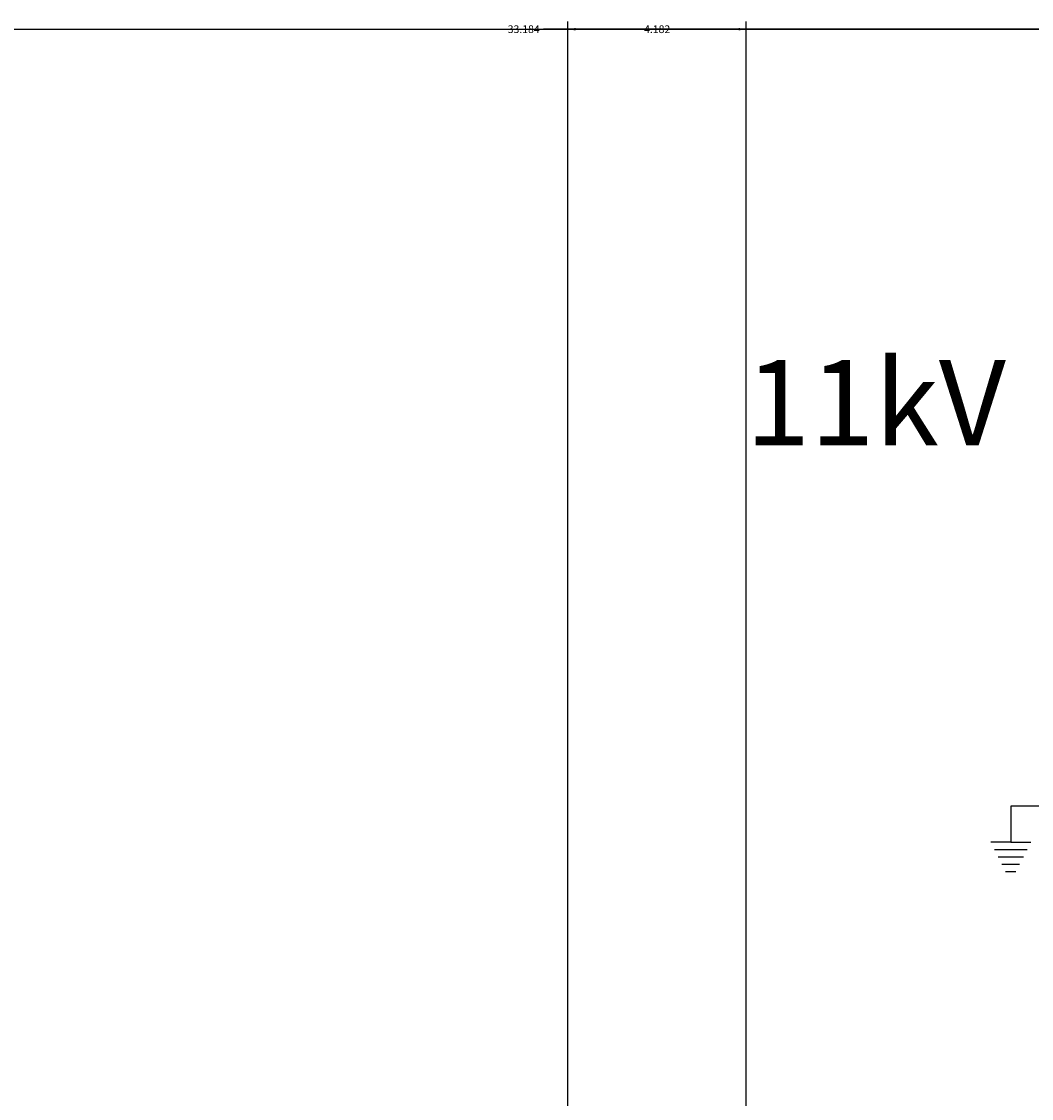
# Model space of a CAD drawing. Units: inches. Extents: x 412 to 584, y 208 to 437.
# Tile 24 of 28: x 471 to 495, y 412 to 437. Entities that reach past the tile are written whole.
import ezdxf

# ---------------------------------------------------------------- set-up
doc = ezdxf.new("R2010")
doc.units = ezdxf.units.IN
doc.header["$MEASUREMENT"] = 0
for name, color, linetype, lineweight in [('A-ANNO-DIMS', 2, 'Continuous', 18), ('E-ANNO-TEXT', 7, 'Continuous', 18), ('E-POWR-EQPM', 3, 'Continuous', 25)]:
    doc.layers.add(name, color=color, linetype=linetype, lineweight=lineweight)
doc.styles.get("Standard").update_dxf_attribs({"font": 'arial.ttf'})
doc.dimstyles.get("Standard").update_dxf_attribs({"dimtxt": 0.18, "dimasz": 0.18, "dimexe": 0.18, "dimexo": 0.0625, "dimgap": 0.09, "dimtad": 0, "dimtih": 1, "dimtoh": 1, "dimdec": 4, "dimzin": 0, "dimdsep": 46, "dimtxsty": 'Standard', "dimcen": 0.09, "dimadec": 0, "dimazin": 0, "dimtfac": 1, "dimtdec": 4, "dimtofl": 0, "dimtmove": 0, "dimatfit": 3, "dimfxl": 1, "dimtolj": 1, "dimtzin": 0, "dimarcsym": 0})

# ---------------------------------------------------------------- blocks, each defined once
blk = doc.blocks.new('*D21')
at = {"layer": 'A-ANNO-DIMS', "color": 0, "lineweight": -2, "transparency": 16777216}
for p, q in [((466.104, 400.237), (466.104, 437.465)), ((538.619, 400.237), (538.619, 437.465)), ((466.284, 437.285), (501.986, 437.285)), ((538.439, 437.285), (502.737, 437.285))]:
    blk.add_line(p, q, dxfattribs=at)
at = {"layer": 'A-ANNO-DIMS', "color": 0, "transparency": 16777216}
for points in [[(466.284, 437.315), (466.284, 437.255), (466.104, 437.285)], [(538.439, 437.315), (538.439, 437.255), (538.619, 437.285)]]:
    blk.add_solid(points, dxfattribs=at)
at = {"layer": 'Defpoints', "color": 0, "transparency": 16777216}
for p in [(538.619, 437.285), (466.104, 400.175), (538.619, 400.175)]:
    blk.add_point(p, dxfattribs=at)
at = {"layer": 'A-ANNO-DIMS', "color": 0, "transparency": 16777216, "insert": (502.361, 437.285), "char_height": 0.18, "attachment_point": 5}
blk.add_mtext('\\A1;72.51', dxfattribs=at)
blk = doc.blocks.new('*D27')
at = {"layer": 'A-ANNO-DIMS', "color": 0, "lineweight": -2, "transparency": 16777216}
for p, q in [((466.104, 400.237), (466.104, 437.465)), ((499.288, 397.825), (499.288, 437.465)), ((466.284, 437.285), (482.233, 437.285)), ((499.108, 437.285), (483.159, 437.285))]:
    blk.add_line(p, q, dxfattribs=at)
at = {"layer": 'A-ANNO-DIMS', "color": 0, "transparency": 16777216}
for points in [[(466.284, 437.315), (466.284, 437.255), (466.104, 437.285)], [(499.108, 437.315), (499.108, 437.255), (499.288, 437.285)]]:
    blk.add_solid(points, dxfattribs=at)
at = {"layer": 'Defpoints', "color": 0, "transparency": 16777216}
for p in [(499.288, 437.285), (466.104, 400.175), (499.288, 397.763)]:
    blk.add_point(p, dxfattribs=at)
at = {"layer": 'A-ANNO-DIMS', "color": 0, "transparency": 16777216, "insert": (482.696, 437.285), "char_height": 0.18, "attachment_point": 5}
blk.add_mtext('\\A1;33.184', dxfattribs=at)
blk = doc.blocks.new('*D28')
at = {"layer": 'A-ANNO-DIMS', "color": 0, "lineweight": -2, "transparency": 16777216}
for p, q in [((450.562, 256.635), (450.562, 437.465)), ((555.796, 256.635), (555.796, 437.465)), ((450.742, 437.285), (502.724, 437.285)), ((555.616, 437.285), (503.634, 437.285))]:
    blk.add_line(p, q, dxfattribs=at)
at = {"layer": 'A-ANNO-DIMS', "color": 0, "transparency": 16777216}
for points in [[(450.742, 437.315), (450.742, 437.255), (450.562, 437.285)], [(555.616, 437.315), (555.616, 437.255), (555.796, 437.285)]]:
    blk.add_solid(points, dxfattribs=at)
at = {"layer": 'Defpoints', "color": 0, "transparency": 16777216}
for p in [(555.796, 437.285), (450.562, 256.573), (555.796, 256.573)]:
    blk.add_point(p, dxfattribs=at)
at = {"layer": 'A-ANNO-DIMS', "color": 0, "transparency": 16777216, "insert": (503.179, 437.285), "char_height": 0.18, "attachment_point": 5}
blk.add_mtext('\\A1;105.23', dxfattribs=at)
blk = doc.blocks.new('*D41')
at = {"layer": 'A-ANNO-DIMS', "color": 0, "lineweight": -2, "transparency": 16777216}
for p, q in [((483.735, 316.045), (483.735, 437.465)), ((487.917, 316.045), (487.917, 437.465)), ((483.915, 437.285), (485.429, 437.285)), ((487.737, 437.285), (486.222, 437.285))]:
    blk.add_line(p, q, dxfattribs=at)
at = {"layer": 'A-ANNO-DIMS', "color": 0, "transparency": 16777216}
for points in [[(483.915, 437.315), (483.915, 437.255), (483.735, 437.285)], [(487.737, 437.315), (487.737, 437.255), (487.917, 437.285)]]:
    blk.add_solid(points, dxfattribs=at)
at = {"layer": 'Defpoints', "color": 0, "transparency": 16777216}
for p in [(487.917, 437.285), (483.735, 315.982), (487.917, 315.982)]:
    blk.add_point(p, dxfattribs=at)
at = {"layer": 'A-ANNO-DIMS', "color": 0, "transparency": 16777216, "insert": (485.826, 437.285), "char_height": 0.18, "attachment_point": 5}
blk.add_mtext('\\A1;4.182', dxfattribs=at)

msp = doc.modelspace()

# ---------------------------------------------------------------- linework, layer by layer
at = {"layer": 'E-POWR-EQPM'}
for p, q in [((495.8126, 419.0552), (494.1202, 419.0552)), ((494.1202, 419.0552), (494.1202, 418.2146)), ((494.1202, 418.2146), (493.651, 418.2146)), ((494.1202, 418.2146), (494.5894, 418.2146)), ((493.7376, 418.0415), (494.5028, 418.0415)), ((493.8241, 417.8683), (494.4162, 417.8683)), ((493.9107, 417.6952), (494.3297, 417.6952)), ((493.9972, 417.5221), (494.2431, 417.5221))]:
    msp.add_line(p, q, dxfattribs=at)

# ---------------------------------------------------------------- texts
at = {"layer": 'E-ANNO-TEXT', "insert": (486.3843, 432.8579), "char_height": 2, "attachment_point": 1}
msp.add_mtext_dynamic_manual_height_columns('\\pxqc;From\\P11kV Incoming Line', width=27.755796, gutter_width=1, heights=[8.8771], dxfattribs=at)

# ---------------------------------------------------------------- dimensions: what is measured, and where the dimension line sits
at = {"layer": 'A-ANNO-DIMS'}
for base, p1, p2, override, picture, middle in [((555.7959, 437.2847), (450.562, 256.5729), (555.7959, 256.5729), {"dimdec": 2, "dimlfac": 1, "dimrnd": 0, "dimzin": 0, "dimdsep": 46, "dimlunit": 2}, '*D28', (503.1789, 437.2847)), ((538.6186, 437.2847), (466.1037, 400.175), (538.6186, 400.175), {"dimdec": 2, "dimlfac": 1, "dimrnd": 0, "dimzin": 0, "dimdsep": 46, "dimlunit": 2}, '*D21', (502.3612, 437.2847)), ((499.2878, 437.2847), (466.1037, 400.175), (499.2878, 397.7626), {"dimdec": 3, "dimlfac": 1, "dimrnd": 0, "dimzin": 0, "dimdsep": 46, "dimlunit": 2}, '*D27', (482.6958, 437.2847)), ((487.9167, 437.2847), (483.7347, 315.9821), (487.9167, 315.9821), {"dimdec": 3, "dimlfac": 1, "dimrnd": 0, "dimzin": 0, "dimdsep": 46, "dimlunit": 2}, '*D41', (485.8257, 437.2847))]:
    dim = msp.add_linear_dim(base=base, p1=p1, p2=p2, dimstyle='Standard', override=override, dxfattribs=at)
    dim.commit()
    dim.dimension.update_dxf_attribs({"geometry": picture, "text_midpoint": middle})

doc.saveas('drawing.dxf')
